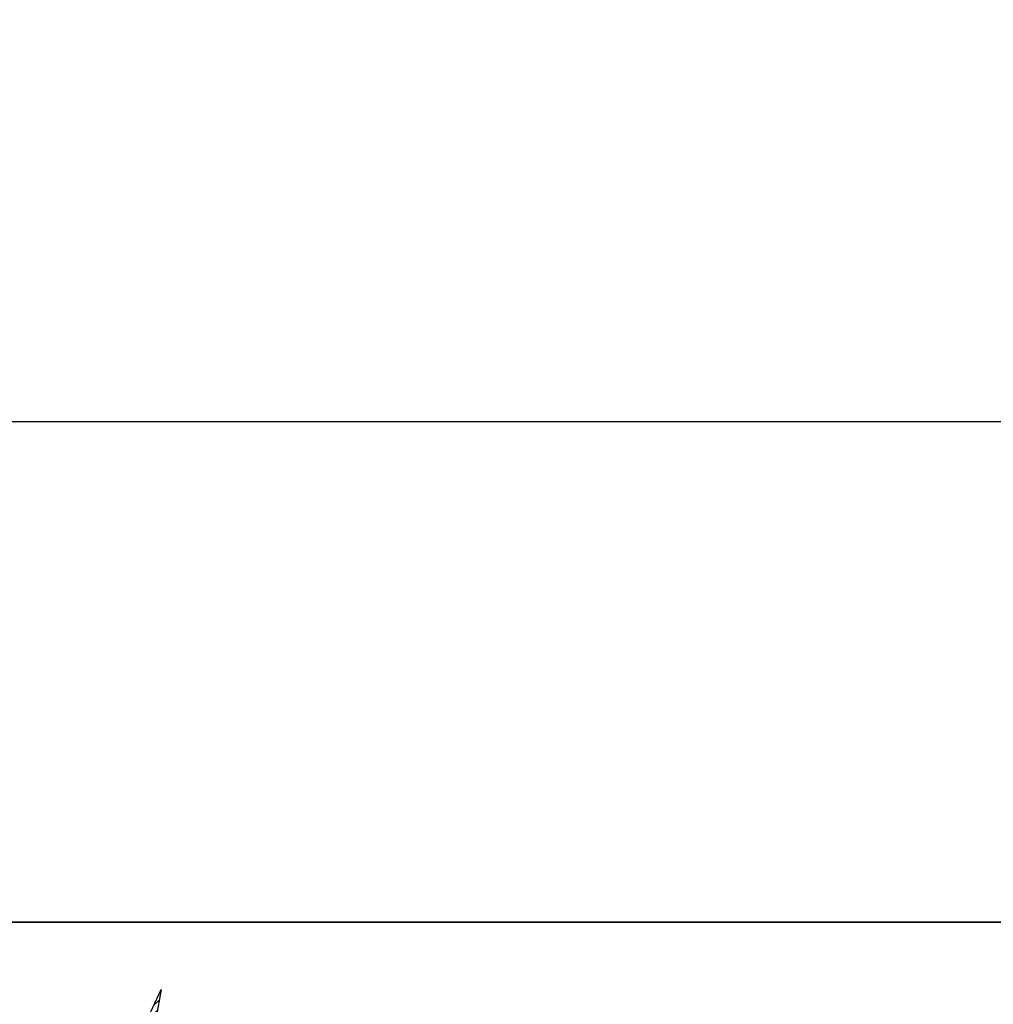
# Model space of a CAD drawing. Units: inches. Extents: x 1986 to 21484, y -1816 to 2016.
# Tile 78 of 85: x 3676 to 3701, y 1899 to 1924. Entities that reach past the tile are written whole.
import ezdxf

# ---------------------------------------------------------------- set-up
doc = ezdxf.new("R2010")
doc.units = ezdxf.units.IN
for name, color, linetype, lineweight in [('A-ANNO-DIMS', 2, 'Continuous', 18), ('C-PROP', 7, 'Continuous', 35), ('L-PLNT', 84, 'Continuous', 13), ('vfolhas', 114, 'Continuous', 5)]:
    doc.layers.add(name, color=color, linetype=linetype, lineweight=lineweight)
doc.layers.add('vfolhas2', color=102, linetype='Continuous')
doc.styles.get("Standard").update_dxf_attribs({"font": 'arial.ttf'})
doc.dimstyles.new('ISO-25', dxfattribs={"dimtxt": 8, "dimasz": 2.5, "dimexe": 1.25, "dimexo": 0.625, "dimtad": 1, "dimdec": 1, "dimlunit": 3, "dimtxsty": 'Standard', "dimcen": 2.5, "dimadec": 0, "dimazin": 0, "dimtfac": 1, "dimtdec": 1, "dimtmove": 0, "dimatfit": 3, "dimfxl": 1, "dimarcsym": 0})

# ---------------------------------------------------------------- blocks, each defined once
blk = doc.blocks.new('*D33')
at = {"layer": 'A-ANNO-DIMS', "color": 0, "lineweight": -2, "transparency": 16777216}
for p, q in [((3538.907, 1901.377), (3538.907, 1914.655)), ((3898.907, 1901.377), (3898.907, 1914.655)), ((3541.407, 1913.405), (3896.407, 1913.405))]:
    blk.add_line(p, q, dxfattribs=at)
at = {"layer": 'A-ANNO-DIMS', "color": 0, "transparency": 16777216}
for points in [[(3541.407, 1913.821), (3541.407, 1912.988), (3538.907, 1913.405)], [(3896.407, 1913.821), (3896.407, 1912.988), (3898.907, 1913.405)]]:
    blk.add_solid(points, dxfattribs=at)
at = {"layer": 'Defpoints', "color": 0, "transparency": 16777216}
for p in [(3898.907, 1913.405), (3538.907, 1900.752), (3898.907, 1900.752)]:
    blk.add_point(p, dxfattribs=at)
at = {"layer": 'A-ANNO-DIMS', "color": 0, "transparency": 16777216, "insert": (3718.907, 1918.117), "char_height": 8, "attachment_point": 5}
blk.add_mtext("30'", dxfattribs=at)
blk = doc.blocks.new('arbusto_PB_verde_grande')
at = {"layer": 'vfolhas'}
h = blk.add_hatch(dxfattribs=at)
h.set_pattern_fill('ANSI31', color=256, scale=0.05, style=0)
h.set_pattern_definition([(45, (-2446.5133113, 50.986076), (-0.004419417382, 0.004419417382), [])])
h.paths.add_polyline_path([(-0.0728, 0.5067), (-0.1808, 0.6506), (-0.2334, 0.6725), (-0.2071, 0.5318), (-0.1078, 0.2501), (0.0263, -0.0393), (0.0003, 0.0905), (0.0082, 0.1624), (-0.0494, 0.2908)])
h.paths.add_polyline_path([(0.099, 0.4193), (0.0937, 0.2657), (0.0791, 0.1881), (0.1551, 0.369), (0.2661, 0.5505), (0.2836, 0.635), (0.2485, 0.6882), (0.2514, 0.635), (0.2018, 0.5443)])
h.paths.add_polyline_path([(0.1229, 0.2407), (0.047, 0.0623), (0.0263, -0.0393), (0.1112, 0.0436), (0.1843, 0.0936), (0.2748, 0.1938), (0.3215, 0.2532), (0.4413, 0.3847), (0.4763, 0.5787), (0.4179, 0.4535), (0.2894, 0.3095)])
h.paths.add_polyline_path([(0.5815, -0.0378), (0.7071, 0.0154), (0.7859, 0.0467), (0.748, 0.0655), (0.6282, 0.0842), (0.526, 0.0905), (0.3974, 0.0436), (0.0263, -0.0393), (0.2573, -0.0315), (0.4383, -0.0347)])
h.paths.add_polyline_path([(0.5202, -0.0365), (0.4383, -0.0347), (0.2573, -0.0315), (0.0263, -0.0393), (0.1796, -0.0852), (0.5377, -0.1317), (0.6954, -0.1536), (0.7859, -0.0785), (0.7041, -0.1004)])
h.paths.add_polyline_path([(0.2719, -0.2193), (0.1492, -0.1411), (0.0263, -0.0393), (0.1579, -0.3101), (0.2952, -0.4258), (0.4179, -0.4916), (0.564, -0.5667), (0.5114, -0.4853), (0.3946, -0.3414)])
h.paths.add_polyline_path([(-0.0582, -0.4759), (-0.0231, -0.6198), (0.047, -0.8013), (0.0849, -0.5979), (0.0791, -0.4071), (0.0353, -0.2538), (0.0263, -0.0393), (-0.0377, -0.26)])
h.paths.add_polyline_path([(-0.2422, 0.1405), (-0.1107, 0.0686), (0.0263, -0.0393), (-0.0423, 0.1087), (-0.2101, 0.2376), (-0.3649, 0.3314), (-0.4787, 0.4034), (-0.543, 0.4629), (-0.4904, 0.3314), (-0.3941, 0.2219)])
at = {"layer": 'vfolhas2'}
for p, q in [((0.4179, 0.4535), (0.4763, 0.5787)), ((0.4763, 0.5787), (0.4413, 0.3847))]:
    blk.add_line(p, q, dxfattribs=at)

msp = doc.modelspace()

# ---------------------------------------------------------------- linework, layer by layer
at = {"layer": 'C-PROP'}
msp.add_lwpolyline([(3538.907, 1900.752), (3898.907, 1900.752), (3898.907, 1066.752), (3538.907, 1066.752)], close=True, dxfattribs=at)

# ---------------------------------------------------------------- block references
at = {"layer": 'L-PLNT', "xscale": 24.60366729364114, "yscale": 24.60366729364114, "zscale": 24.60366729364114}
msp.add_blockref('arbusto_PB_verde_grande', (3668.218, 1884.805), dxfattribs=at)

# ---------------------------------------------------------------- dimensions: what is measured, and where the dimension line sits
at = {"layer": 'A-ANNO-DIMS'}
dim = msp.add_linear_dim(base=(3898.907, 1913.405), p1=(3538.907, 1900.752), p2=(3898.907, 1900.752), dimstyle='ISO-25', override={"dimclrd": 0, "dimclre": 0, "dimclrt": 0}, dxfattribs=at)
dim.commit()
dim.dimension.update_dxf_attribs({"geometry": '*D33', "text_midpoint": (3718.907, 1918.117)})

doc.saveas('drawing.dxf')
